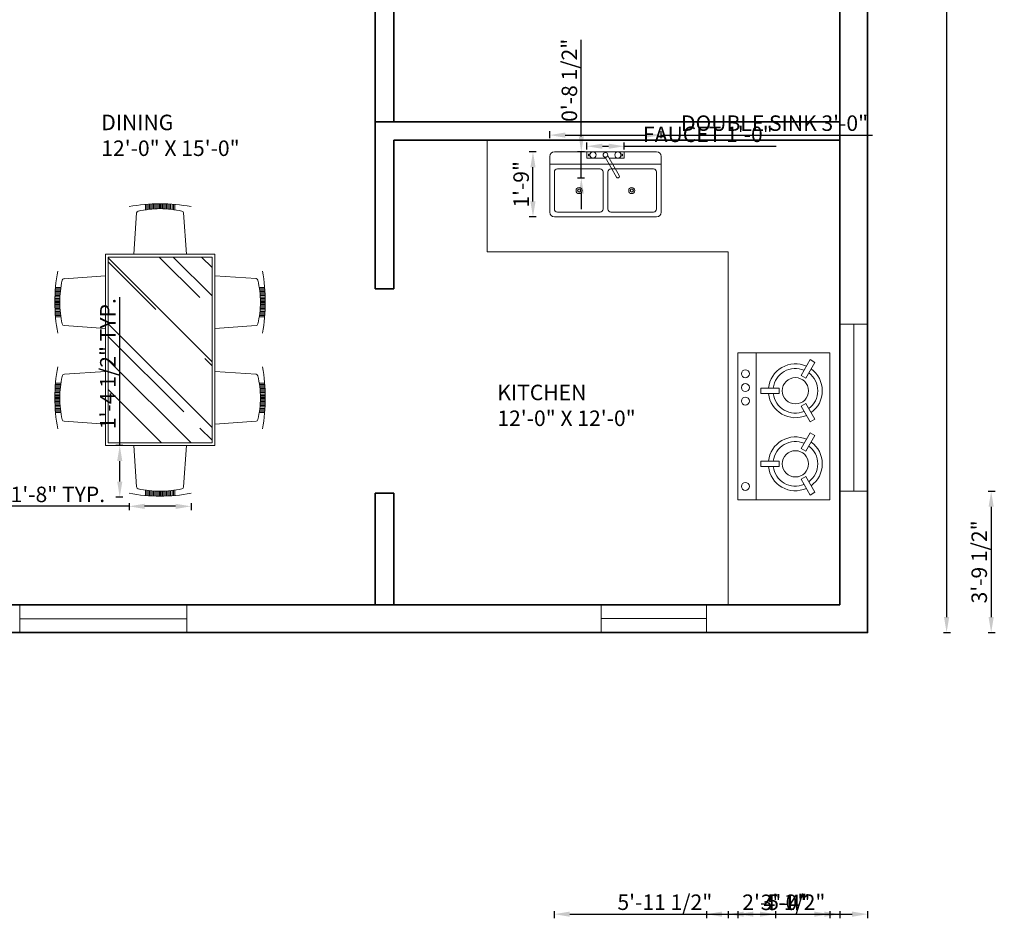
# Model space of a CAD drawing. Units: inches. Extents: x -100 to 766, y -562 to 63.
# Tile 10 of 11: x 448 to 766, y -562 to -269. Entities that reach past the tile are written whole.
import ezdxf

# ---------------------------------------------------------------- set-up
doc = ezdxf.new("R2010")
doc.units = ezdxf.units.IN
for name, color, linetype, lineweight in [('A-ANNO-DIMS', 2, 'Continuous', 18), ('A-AREA-IDEN', 7, 'Continuous', 18), ('A-EQPM', 9, 'Continuous', 18), ('A-FLOR-CASE', 32, 'Continuous', 18), ('A-FLOR-FIXT', 8, 'Continuous', 18), ('A-FURN-PATT', 252, 'Continuous', 13), ('A-GLAZ', 4, 'Continuous', 18), ('A-WALL', 7, 'Continuous', 35), ('furn', 8, 'Continuous', 13)]:
    doc.layers.add(name, color=color, linetype=linetype, lineweight=lineweight)
doc.styles.get("Standard").update_dxf_attribs({"font": 'arial.ttf'})
doc.dimstyles.new('ISO-25', dxfattribs={"dimtxt": 5, "dimasz": 5, "dimexe": 1.25, "dimexo": 0.625, "dimtad": 1, "dimlunit": 3, "dimtxsty": 'Standard', "dimcen": 2.5, "dimadec": 0, "dimazin": 0, "dimtfac": 1, "dimtmove": 0, "dimatfit": 3, "dimfxl": 1, "dimfxlon": 1, "dimarcsym": 0})

# ---------------------------------------------------------------- blocks, each defined once
blk = doc.blocks.new('Sink-double - 36 in top')
for p, q in [((-18, -4), (18, -4)), ((-0.75, -18.5), (-0.75, -6.5)), ((0.75, -6.5), (0.75, -18.5))]:
    blk.add_line(p, q)
for points in [[(-16.5, 0), (16.5, 0)], [(-18, -19.5), (-18, -1.5)], [(18, -1.5), (18, -19.5)], [(-15.5, -5.5), (-1.75, -5.5)], [(1.75, -5.5), (15.5, -5.5)], [(-16.5, -18.5), (-16.5, -6.5)], [(16.5, -6.5), (16.5, -18.5)], [(16.5, -21), (-16.5, -21)], [(-1.75, -19.5), (-15.5, -19.5)], [(15.5, -19.5), (1.75, -19.5)]]:
    blk.add_lwpolyline(points)
for centre, radius in [((-8.5, -12.5), 1), ((-8.5, -12.5), 0.5), ((8.5, -12.5), 1), ((8.5, -12.5), 0.5)]:
    blk.add_circle(centre, radius)
for centre, radius, start, end in [((-16.5, -1.5), 1.5, 90, 180), ((16.5, -1.5), 1.5, 0, 90), ((-15.5, -6.5), 1, 90, 180), ((-1.75, -6.5), 1, 0, 90), ((1.75, -6.5), 1, 90, 180), ((15.5, -6.5), 1, 0, 90), ((-15.5, -18.5), 1, 180, 270), ((-1.75, -18.5), 1, 270, 0), ((1.75, -18.5), 1, 180, 270), ((15.5, -18.5), 1, 270, 0), ((-16.5, -19.5), 1.5, 180, 270), ((16.5, -19.5), 1.5, 270, 0)]:
    blk.add_arc(centre, radius, start, end)
blk = doc.blocks.new('Faucet - kit sink top')
for p, q in [((-5.5, -0.75), (-5.5, -1.25)), ((-4.94278, -0.75), (-5.5, -0.75)), ((-5.5, -1.25), (-4.94278, -1.25)), ((-0.14775, -1.7441), (3.56698, -8.1782)), ((4.43301, -7.6782), (0.71828, -1.2441)), ((4.94278, -0.75), (5.5, -0.75)), ((5.5, -1.25), (4.94278, -1.25)), ((5.5, -0.75), (5.5, -1.25))]:
    blk.add_line(p, q)
blk.add_lwpolyline([(-0.00587, -2), (-6, -2), (-6, 0), (6, 0), (6, -2), (1.15195, -2)])
for centre, radius in [((-4, -1), 1), ((4, -1), 1), ((0, -1), 0.75)]:
    blk.add_circle(centre, radius)
blk.add_arc((4, -7.9282), 0.5, 210, 30)
blk = doc.blocks.new('*D10')
at = {"layer": 'A-ANNO-DIMS', "color": 0, "lineweight": -2, "transparency": 16777216}
for p, q in [((745.89, 12.79), (748.14, 12.79)), ((746.89, 7.79), (746.89, -462.21)), ((745.89, -467.21), (748.14, -467.21))]:
    blk.add_line(p, q, dxfattribs=at)
at = {"layer": 'A-ANNO-DIMS', "color": 0, "transparency": 16777216}
for points in [[(746.06, 7.79), (747.73, 7.79), (746.89, 12.79)], [(746.06, -462.21), (747.73, -462.21), (746.89, -467.21)]]:
    blk.add_solid(points, dxfattribs=at)
at = {"layer": 'Defpoints', "color": 0, "transparency": 16777216}
for p in [(721.39, 12.79), (721.39, -467.21), (746.89, -467.21)]:
    blk.add_point(p, dxfattribs=at)
at = {"layer": 'A-ANNO-DIMS', "color": 0, "transparency": 16777216, "insert": (743.72, -227.21), "char_height": 5, "attachment_point": 5, "rotation": 90}
blk.add_mtext("40'", dxfattribs=at)
blk = doc.blocks.new('WIN-54IN')
blk.add_line((4.5, 54), (4.5, 0))
blk.add_lwpolyline([(0, 54), (9, 54), (9, 0), (0, 0)], close=True)
blk = doc.blocks.new('WIN-34IN')
blk.add_line((4.5, 34), (4.5, 0))
blk.add_lwpolyline([(0, 34), (9, 34), (9, 0), (0, 0)], close=True)
blk = doc.blocks.new('CHAIR-DINING')
for p, q in [((16.31, 18.5), (2.96, 17.59)), ((1.73, 12.99), (0.08, 12.99)), ((1.77, 13.43), (0.11, 13.43)), ((1.83, 13.87), (0.13, 13.87)), ((1.88, 14.32), (0.17, 14.32)), ((1.94, 14.76), (0.2, 14.76)), ((1.56, 10.34), (0, 10.34)), ((1.56, 10.01), (0, 10.01)), ((1.56, 9.68), (0, 9.68)), ((1.6, 11.23), (0.01, 11.23)), ((1.58, 10.79), (0.01, 10.79)), ((1.62, 11.67), (0.02, 11.67)), ((1.65, 12.11), (0.04, 12.11)), ((1.69, 12.55), (0.06, 12.55)), ((1.58, 9.24), (0.01, 9.24)), ((1.6, 8.8), (0.01, 8.8)), ((1.62, 8.36), (0.02, 8.36)), ((1.65, 7.92), (0.04, 7.92)), ((1.69, 7.48), (0.06, 7.48)), ((1.73, 7.04), (0.08, 7.04)), ((1.77, 6.6), (0.11, 6.6)), ((1.83, 6.15), (0.13, 6.15)), ((1.88, 5.71), (0.17, 5.71)), ((1.94, 5.27), (0.2, 5.27)), ((16.31, 1.53), (2.96, 2.43))]:
    blk.add_line(p, q)
blk.add_lwpolyline([(0.91, 20.03, 0.091245), (0.91, 0, 0.091245)], format="xyb")
for centre, radius, start, end in [((38.68, 9.38), 37.13, 168.0355, 179.0138), ((3.01, 16.93), 0.662, 93.8745, 168.0355), ((38.68, 10.65), 37.13, 180.9862, 191.9645), ((3.01, 3.09), 0.662, 191.9645, 266.1255)]:
    blk.add_arc(centre, radius, start, end)
blk = doc.blocks.new('*D24')
at = {"layer": 'A-ANNO-DIMS', "color": 0, "lineweight": -2, "transparency": 16777216}
for p, q in [((482.94, -425.44), (482.94, -427.69)), ((502.97, -425.44), (502.97, -427.69)), ((482.94, -426.44), (404.32, -426.44)), ((497.97, -426.44), (487.94, -426.44))]:
    blk.add_line(p, q, dxfattribs=at)
at = {"layer": 'A-ANNO-DIMS', "color": 0, "transparency": 16777216}
for points in [[(487.94, -425.61), (487.94, -427.28), (482.94, -426.44)], [(497.97, -425.61), (497.97, -427.28), (502.97, -426.44)]]:
    blk.add_solid(points, dxfattribs=at)
at = {"layer": 'Defpoints', "color": 0, "transparency": 16777216}
for p in [(482.94, -423.44), (502.97, -423.44), (482.94, -426.44)]:
    blk.add_point(p, dxfattribs=at)
at = {"layer": 'A-ANNO-DIMS', "color": 0, "transparency": 16777216, "insert": (441.13, -423.23), "char_height": 5, "attachment_point": 5, "rotation": 0}
blk.add_mtext('SIDE CHAIR 1\'-8" TYP.', dxfattribs=at)
blk = doc.blocks.new('*D25')
at = {"layer": 'A-ANNO-DIMS', "color": 0, "lineweight": -2, "transparency": 16777216}
for p, q in [((479.93, -406.82), (479.93, -358.91)), ((480.93, -406.82), (478.68, -406.82)), ((479.93, -418.44), (479.93, -411.82)), ((480.93, -423.44), (478.68, -423.44))]:
    blk.add_line(p, q, dxfattribs=at)
at = {"layer": 'A-ANNO-DIMS', "color": 0, "transparency": 16777216}
for points in [[(479.1, -411.82), (480.77, -411.82), (479.93, -406.82)], [(479.1, -418.44), (480.77, -418.44), (479.93, -423.44)]]:
    blk.add_solid(points, dxfattribs=at)
at = {"layer": 'Defpoints', "color": 0, "transparency": 16777216}
for p in [(479.93, -406.82), (482.94, -406.82), (482.94, -423.44)]:
    blk.add_point(p, dxfattribs=at)
at = {"layer": 'A-ANNO-DIMS', "color": 0, "transparency": 16777216, "insert": (476.72, -380.37), "char_height": 5, "attachment_point": 5, "rotation": 90}
blk.add_mtext('1\'-4 1/2" TYP.', dxfattribs=at)
blk = doc.blocks.new('*D36')
at = {"layer": 'A-ANNO-DIMS', "color": 0, "lineweight": -2, "transparency": 16777216}
for p, q in [((630.75, -311.15), (630.75, -308.9)), ((635.75, -310.15), (637.75, -310.15)), ((642.75, -311.15), (642.75, -308.9)), ((642.75, -310.15), (691.89, -310.15))]:
    blk.add_line(p, q, dxfattribs=at)
at = {"layer": 'A-ANNO-DIMS', "color": 0, "transparency": 16777216}
for points in [[(635.75, -309.31), (635.75, -310.98), (630.75, -310.15)], [(637.75, -309.31), (637.75, -310.98), (642.75, -310.15)]]:
    blk.add_solid(points, dxfattribs=at)
at = {"layer": 'Defpoints', "color": 0, "transparency": 16777216}
for p in [(642.75, -310.15), (630.75, -311.95), (642.75, -311.95)]:
    blk.add_point(p, dxfattribs=at)
at = {"layer": 'A-ANNO-DIMS', "color": 0, "transparency": 16777216, "insert": (669.82, -306.94), "char_height": 5, "attachment_point": 5}
blk.add_mtext('FAUCET 1\'-0"', dxfattribs=at)
blk = doc.blocks.new('*D37')
at = {"layer": 'A-ANNO-DIMS', "color": 0, "lineweight": -2, "transparency": 16777216}
for p, q in [((628.95, -306.95), (628.95, -275.75)), ((629.95, -311.95), (627.7, -311.95)), ((628.95, -320.45), (628.95, -311.95)), ((629.95, -320.45), (627.7, -320.45)), ((628.95, -325.45), (628.95, -330.45))]:
    blk.add_line(p, q, dxfattribs=at)
at = {"layer": 'A-ANNO-DIMS', "color": 0, "transparency": 16777216}
for points in [[(628.12, -306.95), (629.78, -306.95), (628.95, -311.95)], [(628.12, -325.45), (629.78, -325.45), (628.95, -320.45)]]:
    blk.add_solid(points, dxfattribs=at)
at = {"layer": 'Defpoints', "color": 0, "transparency": 16777216}
for p in [(628.95, -311.95), (630.75, -311.95), (630.75, -320.45)]:
    blk.add_point(p, dxfattribs=at)
at = {"layer": 'A-ANNO-DIMS', "color": 0, "transparency": 16777216, "insert": (625.74, -288.85), "char_height": 5, "attachment_point": 5, "rotation": 90}
blk.add_mtext('0\'-8 1/2"', dxfattribs=at)
blk = doc.blocks.new('*D38')
at = {"layer": 'A-ANNO-DIMS', "color": 0, "lineweight": -2, "transparency": 16777216}
for p, q in [((618.75, -307.55), (618.75, -305.3)), ((623.75, -306.55), (649.75, -306.55)), ((654.75, -307.55), (654.75, -305.3)), ((654.75, -306.55), (722.95, -306.55))]:
    blk.add_line(p, q, dxfattribs=at)
at = {"layer": 'A-ANNO-DIMS', "color": 0, "transparency": 16777216}
for points in [[(623.75, -305.71), (623.75, -307.38), (618.75, -306.55)], [(649.75, -305.71), (649.75, -307.38), (654.75, -306.55)]]:
    blk.add_solid(points, dxfattribs=at)
at = {"layer": 'Defpoints', "color": 0, "transparency": 16777216}
for p in [(654.75, -306.55), (618.75, -311.95), (654.75, -311.95)]:
    blk.add_point(p, dxfattribs=at)
at = {"layer": 'A-ANNO-DIMS', "color": 0, "transparency": 16777216, "insert": (691.35, -303.33), "char_height": 5, "attachment_point": 5}
blk.add_mtext('DOUBLE SINK 3\'-0"', dxfattribs=at)
blk = doc.blocks.new('*D39')
at = {"layer": 'A-ANNO-DIMS', "color": 0, "lineweight": -2, "transparency": 16777216}
for p, q in [((614.35, -311.95), (612.1, -311.95)), ((613.35, -327.95), (613.35, -316.95)), ((614.35, -332.95), (612.1, -332.95))]:
    blk.add_line(p, q, dxfattribs=at)
at = {"layer": 'A-ANNO-DIMS', "color": 0, "transparency": 16777216}
for points in [[(612.52, -316.95), (614.18, -316.95), (613.35, -311.95)], [(612.52, -327.95), (614.18, -327.95), (613.35, -332.95)]]:
    blk.add_solid(points, dxfattribs=at)
at = {"layer": 'Defpoints', "color": 0, "transparency": 16777216}
for p in [(613.35, -311.95), (618.75, -311.95), (618.75, -332.95)]:
    blk.add_point(p, dxfattribs=at)
at = {"layer": 'A-ANNO-DIMS', "color": 0, "transparency": 16777216, "insert": (610.17, -322.45), "char_height": 5, "attachment_point": 5, "rotation": 90}
blk.add_mtext('1\'-9"', dxfattribs=at)
blk = doc.blocks.new('*D49')
at = {"layer": 'A-ANNO-DIMS', "color": 0, "lineweight": -2, "transparency": 16777216}
for p, q in [((-88.51, -356.21), (-90.76, -356.21)), ((-89.51, -361.21), (-89.51, -417.21)), ((-88.51, -422.21), (-90.76, -422.21))]:
    blk.add_line(p, q, dxfattribs=at)
at = {"layer": 'A-ANNO-DIMS', "color": 0, "transparency": 16777216}
for points in [[(-90.35, -361.21), (-88.68, -361.21), (-89.51, -356.21)], [(-90.35, -417.21), (-88.68, -417.21), (-89.51, -422.21)]]:
    blk.add_solid(points, dxfattribs=at)
at = {"layer": 'Defpoints', "color": 0, "transparency": 16777216}
for p in [(562.39, -356.21), (-89.51, -422.21), (562.39, -422.21)]:
    blk.add_point(p, dxfattribs=at)
at = {"layer": 'A-ANNO-DIMS', "color": 0, "transparency": 16777216, "insert": (-92.69, -389.21), "char_height": 5, "attachment_point": 5, "rotation": 90}
blk.add_mtext('5\'-6"', dxfattribs=at)
blk = doc.blocks.new('*D50')
at = {"layer": 'A-ANNO-DIMS', "color": 0, "lineweight": -2, "transparency": 16777216}
for p, q in [((676.39, -557.16), (676.39, -559.41)), ((681.39, -558.16), (707.39, -558.16)), ((712.39, -557.16), (712.39, -559.41))]:
    blk.add_line(p, q, dxfattribs=at)
at = {"layer": 'A-ANNO-DIMS', "color": 0, "transparency": 16777216}
for points in [[(681.39, -557.32), (681.39, -558.99), (676.39, -558.16)], [(707.39, -557.32), (707.39, -558.99), (712.39, -558.16)]]:
    blk.add_solid(points, dxfattribs=at)
at = {"layer": 'Defpoints', "color": 0, "transparency": 16777216}
for p in [(676.39, -458.21), (712.39, -458.21), (712.39, -558.16)]:
    blk.add_point(p, dxfattribs=at)
at = {"layer": 'A-ANNO-DIMS', "color": 0, "transparency": 16777216, "insert": (694.39, -554.98), "char_height": 5, "attachment_point": 5}
blk.add_mtext('3\'-0"', dxfattribs=at)
blk = doc.blocks.new('*D51')
at = {"layer": 'A-ANNO-DIMS', "color": 0, "lineweight": -2, "transparency": 16777216}
for p, q in [((-88.51, -308.21), (-90.76, -308.21)), ((-89.51, -313.21), (-89.51, -339.21)), ((-88.51, -344.21), (-90.76, -344.21))]:
    blk.add_line(p, q, dxfattribs=at)
at = {"layer": 'A-ANNO-DIMS', "color": 0, "transparency": 16777216}
for points in [[(-90.35, -313.21), (-88.68, -313.21), (-89.51, -308.21)], [(-90.35, -339.21), (-88.68, -339.21), (-89.51, -344.21)]]:
    blk.add_solid(points, dxfattribs=at)
at = {"layer": 'Defpoints', "color": 0, "transparency": 16777216}
for p in [(598.6, -308.21), (-89.51, -344.21), (598.6, -344.21)]:
    blk.add_point(p, dxfattribs=at)
at = {"layer": 'A-ANNO-DIMS', "color": 0, "transparency": 16777216, "insert": (-92.69, -326.21), "char_height": 5, "attachment_point": 5, "rotation": 90}
blk.add_mtext('3\'-0"', dxfattribs=at)
blk = doc.blocks.new('*D52')
at = {"layer": 'A-ANNO-DIMS', "color": 0, "lineweight": -2, "transparency": 16777216}
for p, q in [((568.39, 51.68), (568.39, 53.93)), ((573.39, 52.68), (593.6, 52.68)), ((598.6, 51.68), (598.6, 53.93))]:
    blk.add_line(p, q, dxfattribs=at)
at = {"layer": 'A-ANNO-DIMS', "color": 0, "transparency": 16777216}
for points in [[(573.39, 53.51), (573.39, 51.84), (568.39, 52.68)], [(593.6, 53.51), (593.6, 51.84), (598.6, 52.68)]]:
    blk.add_solid(points, dxfattribs=at)
at = {"layer": 'Defpoints', "color": 0, "transparency": 16777216}
for p in [(598.6, 52.68), (568.39, -308.21), (598.6, -308.21)]:
    blk.add_point(p, dxfattribs=at)
at = {"layer": 'A-ANNO-DIMS', "color": 0, "transparency": 16777216, "insert": (583.5, 55.86), "char_height": 5, "attachment_point": 5}
blk.add_mtext('2\'-6"', dxfattribs=at)
blk = doc.blocks.new('*D64')
at = {"layer": 'A-ANNO-DIMS', "color": 0, "lineweight": -2, "transparency": 16777216}
for p, q in [((760.28, -421.57), (762.53, -421.57)), ((761.28, -426.57), (761.28, -462.21)), ((760.28, -467.21), (762.53, -467.21))]:
    blk.add_line(p, q, dxfattribs=at)
at = {"layer": 'A-ANNO-DIMS', "color": 0, "transparency": 16777216}
for points in [[(760.45, -426.57), (762.11, -426.57), (761.28, -421.57)], [(760.45, -462.21), (762.11, -462.21), (761.28, -467.21)]]:
    blk.add_solid(points, dxfattribs=at)
at = {"layer": 'Defpoints', "color": 0, "transparency": 16777216}
for p in [(721.39, -421.57), (721.39, -467.21), (761.28, -467.21)]:
    blk.add_point(p, dxfattribs=at)
at = {"layer": 'A-ANNO-DIMS', "color": 0, "transparency": 16777216, "insert": (758.07, -444.39), "char_height": 5, "attachment_point": 5, "rotation": 90}
blk.add_mtext('3\'-9 1/2"', dxfattribs=at)
blk = doc.blocks.new('*D69')
at = {"layer": 'A-ANNO-DIMS', "color": 0, "lineweight": -2, "transparency": 16777216}
for p, q in [((669.37, -557.16), (669.37, -559.41)), ((674.37, -558.16), (716.39, -558.16)), ((721.39, -557.16), (721.39, -559.41))]:
    blk.add_line(p, q, dxfattribs=at)
at = {"layer": 'A-ANNO-DIMS', "color": 0, "transparency": 16777216}
for points in [[(674.37, -557.32), (674.37, -558.99), (669.37, -558.16)], [(716.39, -557.32), (716.39, -558.99), (721.39, -558.16)]]:
    blk.add_solid(points, dxfattribs=at)
at = {"layer": 'Defpoints', "color": 0, "transparency": 16777216}
for p in [(669.37, -467.21), (721.39, -467.21), (721.39, -558.16)]:
    blk.add_point(p, dxfattribs=at)
at = {"layer": 'A-ANNO-DIMS', "color": 0, "transparency": 16777216, "insert": (695.38, -555.03), "char_height": 5, "attachment_point": 5}
blk.add_mtext('4\'-4"', dxfattribs=at)
blk = doc.blocks.new('*D70')
at = {"layer": 'A-ANNO-DIMS', "color": 0, "lineweight": -2, "transparency": 16777216}
for p, q in [((-88.51, -376.85), (-90.76, -376.85)), ((-89.51, -381.85), (-89.51, -419.34)), ((-88.51, -424.34), (-90.76, -424.34))]:
    blk.add_line(p, q, dxfattribs=at)
at = {"layer": 'A-ANNO-DIMS', "color": 0, "transparency": 16777216}
for points in [[(-90.35, -381.85), (-88.68, -381.85), (-89.51, -376.85)], [(-90.35, -419.34), (-88.68, -419.34), (-89.51, -424.34)]]:
    blk.add_solid(points, dxfattribs=at)
at = {"layer": 'Defpoints', "color": 0, "transparency": 16777216}
for p in [(679.5, -376.85), (-89.51, -424.34), (679.5, -424.34)]:
    blk.add_point(p, dxfattribs=at)
at = {"layer": 'A-ANNO-DIMS', "color": 0, "transparency": 16777216, "insert": (-92.73, -400.59), "char_height": 5, "attachment_point": 5, "rotation": 90}
blk.add_mtext('3\'-11 1/2"', dxfattribs=at)
blk = doc.blocks.new('*D71')
at = {"layer": 'A-ANNO-DIMS', "color": 0, "lineweight": -2, "transparency": 16777216}
for p, q in [((679.5, -557.16), (679.5, -559.41)), ((684.5, -558.16), (704.17, -558.16)), ((709.17, -557.16), (709.17, -559.41))]:
    blk.add_line(p, q, dxfattribs=at)
at = {"layer": 'A-ANNO-DIMS', "color": 0, "transparency": 16777216}
for points in [[(684.5, -557.32), (684.5, -558.99), (679.5, -558.16)], [(704.17, -557.32), (704.17, -558.99), (709.17, -558.16)]]:
    blk.add_solid(points, dxfattribs=at)
at = {"layer": 'Defpoints', "color": 0, "transparency": 16777216}
for p in [(679.5, -424.34), (709.17, -424.34), (709.17, -558.16)]:
    blk.add_point(p, dxfattribs=at)
at = {"layer": 'A-ANNO-DIMS', "color": 0, "transparency": 16777216, "insert": (694.34, -554.95), "char_height": 5, "attachment_point": 5}
blk.add_mtext('2\'-5 1/2"', dxfattribs=at)
blk = doc.blocks.new('*D72')
at = {"layer": 'A-ANNO-DIMS', "color": 0, "lineweight": -2, "transparency": 16777216}
for p, q in [((475.3, 51.68), (475.3, 53.93)), ((480.3, 52.68), (505.6, 52.68)), ((510.6, 51.68), (510.6, 53.93))]:
    blk.add_line(p, q, dxfattribs=at)
at = {"layer": 'A-ANNO-DIMS', "color": 0, "transparency": 16777216}
for points in [[(480.3, 53.51), (480.3, 51.84), (475.3, 52.68)], [(505.6, 53.51), (505.6, 51.84), (510.6, 52.68)]]:
    blk.add_solid(points, dxfattribs=at)
at = {"layer": 'Defpoints', "color": 0, "transparency": 16777216}
for p in [(510.6, 52.68), (475.3, -345.04), (510.6, -345.04)]:
    blk.add_point(p, dxfattribs=at)
at = {"layer": 'A-ANNO-DIMS', "color": 0, "transparency": 16777216, "insert": (492.95, 55.89), "char_height": 5, "attachment_point": 5}
blk.add_mtext('2\'-11 1/2"', dxfattribs=at)
blk = doc.blocks.new('*D73')
at = {"layer": 'A-ANNO-DIMS', "color": 0, "lineweight": -2, "transparency": 16777216}
for p, q in [((-88.51, -345.04), (-90.76, -345.04)), ((-89.51, -350.04), (-89.51, -401.82)), ((-88.51, -406.82), (-90.76, -406.82))]:
    blk.add_line(p, q, dxfattribs=at)
at = {"layer": 'A-ANNO-DIMS', "color": 0, "transparency": 16777216}
for points in [[(-90.35, -350.04), (-88.68, -350.04), (-89.51, -345.04)], [(-90.35, -401.82), (-88.68, -401.82), (-89.51, -406.82)]]:
    blk.add_solid(points, dxfattribs=at)
at = {"layer": 'Defpoints', "color": 0, "transparency": 16777216}
for p in [(475.3, -345.04), (-89.51, -406.82), (475.3, -406.82)]:
    blk.add_point(p, dxfattribs=at)
at = {"layer": 'A-ANNO-DIMS', "color": 0, "transparency": 16777216, "insert": (-92.69, -375.93), "char_height": 5, "attachment_point": 5, "rotation": 90}
blk.add_mtext('5\'-2"', dxfattribs=at)
blk = doc.blocks.new('*D74')
at = {"layer": 'A-ANNO-DIMS', "color": 0, "lineweight": -2, "transparency": 16777216}
for p, q in [((620.21, -557.16), (620.21, -559.41)), ((625.21, -558.16), (686.63, -558.16)), ((691.63, -557.16), (691.63, -559.41))]:
    blk.add_line(p, q, dxfattribs=at)
at = {"layer": 'A-ANNO-DIMS', "color": 0, "transparency": 16777216}
for points in [[(625.21, -557.32), (625.21, -558.99), (620.21, -558.16)], [(686.63, -557.32), (686.63, -558.99), (691.63, -558.16)]]:
    blk.add_solid(points, dxfattribs=at)
at = {"layer": 'Defpoints', "color": 0, "transparency": 16777216}
for p in [(620.21, -98.08), (691.63, -98.08), (691.63, -558.16)]:
    blk.add_point(p, dxfattribs=at)
at = {"layer": 'A-ANNO-DIMS', "color": 0, "transparency": 16777216, "insert": (655.92, -554.95), "char_height": 5, "attachment_point": 5}
blk.add_mtext('5\'-11 1/2"', dxfattribs=at)
blk = doc.blocks.new('*D83')
at = {"layer": 'A-ANNO-DIMS', "color": 0, "lineweight": -2, "transparency": 16777216}
for p, q in [((-88.51, -422.21), (-90.76, -422.21)), ((-89.51, -427.21), (-89.51, -453.21)), ((-88.51, -458.21), (-90.76, -458.21))]:
    blk.add_line(p, q, dxfattribs=at)
at = {"layer": 'A-ANNO-DIMS', "color": 0, "transparency": 16777216}
for points in [[(-90.35, -427.21), (-88.68, -427.21), (-89.51, -422.21)], [(-90.35, -453.21), (-88.68, -453.21), (-89.51, -458.21)]]:
    blk.add_solid(points, dxfattribs=at)
at = {"layer": 'Defpoints', "color": 0, "transparency": 16777216}
for p in [(562.39, -422.21), (-89.51, -458.21), (562.39, -458.21)]:
    blk.add_point(p, dxfattribs=at)
at = {"layer": 'A-ANNO-DIMS', "color": 0, "transparency": 16777216, "insert": (-92.69, -440.21), "char_height": 5, "attachment_point": 5, "rotation": 90}
blk.add_mtext('3\'-0"', dxfattribs=at)

msp = doc.modelspace()

# ---------------------------------------------------------------- hatches: boundary and pattern name
at = {"layer": 'A-FURN-PATT'}
h = msp.add_hatch(dxfattribs=at)
h.set_pattern_fill('AR-RROOF', color=256, scale=0.882529, angle=-45, style=0)
h.set_pattern_definition([(315, (-259.83, 1276.079), (50.72213, -19.0208), [336.2434, -44.8325, 112.0811, -22.4162]), (315, (-230.824, 1262.923), (5.2307, 36.93205), [67.2487, -7.3974, 134.4974, -16.8122]), (315, (-238.432, 1281.626), (93.04341, -71.80352), [179.3298, -31.3827, 89.6649, -22.4162])])
h.paths.add_polyline_path([(509.719, -345.927), (476.183, -345.927), (476.183, -405.939), (509.719, -405.939)])

# ---------------------------------------------------------------- linework, layer by layer
at = {"layer": 'A-EQPM'}
for p, q in [((679.495, -424.336), (679.495, -376.848)), ((679.495, -376.848), (709.175, -376.848)), ((685.431, -424.336), (685.431, -376.848)), ((709.175, -424.336), (709.175, -376.848)), ((699.899, -384.177), (702.859, -379.055)), ((701.441, -385.068), (704.401, -379.946)), ((702.859, -379.055), (704.401, -379.946)), ((699.899, -384.177), (701.441, -385.068)), ((686.958, -390.008), (686.959, -388.227)), ((692.873, -390.01), (686.958, -390.008)), ((692.874, -388.229), (686.959, -388.227)), ((692.873, -390.01), (692.874, -388.229)), ((701.438, -393.178), (699.896, -394.068)), ((699.896, -394.068), (702.852, -399.192)), ((701.438, -393.178), (704.394, -398.302)), ((704.394, -398.302), (702.852, -399.192)), ((699.899, -407.776), (702.859, -402.654)), ((701.441, -408.667), (704.401, -403.545)), ((702.859, -402.654), (704.401, -403.545)), ((699.899, -407.776), (701.441, -408.667)), ((686.958, -413.607), (686.959, -411.826)), ((692.874, -411.828), (686.959, -411.826)), ((692.873, -413.609), (692.874, -411.828)), ((692.873, -413.609), (686.958, -413.607)), ((701.438, -416.777), (699.896, -417.667)), ((699.896, -417.667), (702.852, -422.791)), ((701.438, -416.777), (704.394, -421.901)), ((704.394, -421.901), (702.852, -422.791)), ((679.495, -424.336), (709.175, -424.336))]:
    msp.add_line(p, q, dxfattribs=at)
at = {"layer": 'A-EQPM', "extrusion": (0, 0, -1)}
for centre, major_axis, start_param, end_param in [((698.07, -389.121), (8.697, 0.005), 3.2450997, 5.1343764), ((681.926, -383.607), (0.911, 0.911), 2.3561945, 8.6393798), ((698.07, -389.121), (5.1, 5.1), 4.0511235, 5.8980015), ((698.07, -389.121), (3.002, 3.002), 2.3561945, 8.6393798), ((698.07, -389.121), (5.1, 5.1), 6.1455186, 7.9923966), ((698.07, -389.121), (8.697, 0.015), -0.9425843, 0.9466925), ((681.926, -388.069), (0.911, 0.911), 2.3561945, 8.6393798), ((698.07, -389.121), (8.697, -0.012), 1.148752, 3.0380287), ((698.07, -389.121), (5.1, -5.1), 0.385932, 2.2328101), ((681.926, -392.432), (0.911, 0.911), 2.3561945, 8.6393798), ((698.07, -412.721), (8.697, -0.003), 3.2441732, 5.1334499), ((698.07, -412.721), (5.1, -5.1), 2.4803271, 4.3272052), ((698.07, -412.721), (8.697, 0.002), -0.9440105, 0.9452662), ((698.07, -412.721), (3.002, 3.002), 2.3561945, 8.6393798), ((698.07, -412.721), (5.1, 5.1), 6.1455186, 7.9923966), ((698.07, -412.721), (8.697, -0.012), 1.1487904, 3.0380671), ((698.07, -412.721), (5.1, -5.1), 0.385932, 2.2328101), ((681.926, -419.997), (0.911, 0.911), 2.3561945, 8.6393798)]:
    msp.add_ellipse(centre, major_axis=major_axis, ratio=1, start_param=start_param, end_param=end_param, dxfattribs=at)
at = {"layer": 'A-FLOR-CASE'}
for p, q in [((598.603, -344.214), (598.603, -308.214)), ((598.603, -344.214), (676.388, -344.214)), ((676.388, -458.214), (676.388, -344.214))]:
    msp.add_line(p, q, dxfattribs=at)
at = {"layer": 'A-WALL'}
for p, q in [((712.388, 3.786), (712.388, -458.214)), ((562.394, -302.214), (562.394, -257.081)), ((568.394, -302.214), (568.394, -257.214)), ((562.394, -306.262), (562.394, -302.214)), ((568.394, -302.214), (562.394, -302.214)), ((712.388, -302.214), (568.394, -302.214)), ((562.394, -312.262), (562.394, -306.262)), ((712.388, -308.214), (568.394, -308.214)), ((568.394, -356.214), (568.394, -308.214)), ((562.394, -356.214), (562.394, -312.262)), ((568.394, -356.214), (562.394, -356.214)), ((562.394, -458.214), (562.394, -422.214)), ((568.394, -422.214), (562.394, -422.214)), ((568.394, -458.214), (568.394, -422.214)), ((532.388, -458.214), (250.388, -458.214)), ((568.394, -458.214), (532.388, -458.214)), ((712.388, -458.214), (568.394, -458.214))]:
    msp.add_line(p, q, dxfattribs=at)
msp.add_lwpolyline([(1.388, 12.786), (721.388, 12.786), (721.388, -467.214), (1.388, -467.214)], close=True, dxfattribs=at)
at = {"layer": 'furn'}
for p, q in [((475.3, -382.892), (462.115, -383.785)), ((460.813, -387.517), (459.122, -387.517)), ((460.869, -387.076), (459.154, -387.076)), ((460.931, -386.635), (459.191, -386.635)), ((460.566, -390.606), (458.992, -390.606)), ((460.585, -390.165), (459, -390.165)), ((460.61, -389.724), (459.012, -389.724)), ((460.64, -389.283), (459.027, -389.283)), ((460.675, -388.841), (459.045, -388.841)), ((460.716, -388.4), (459.067, -388.4)), ((460.762, -387.959), (459.093, -387.959)), ((460.545, -391.377), (458.987, -391.377)), ((460.552, -391.048), (458.988, -391.048)), ((460.552, -391.707), (458.988, -391.707)), ((460.566, -392.149), (458.992, -392.149)), ((460.585, -392.59), (459, -392.59)), ((460.61, -393.031), (459.012, -393.031)), ((460.64, -393.472), (459.027, -393.472)), ((460.675, -393.914), (459.045, -393.914)), ((460.716, -394.355), (459.067, -394.355)), ((460.762, -394.796), (459.093, -394.796)), ((460.813, -395.237), (459.122, -395.237)), ((460.869, -395.679), (459.154, -395.679)), ((460.931, -396.12), (459.191, -396.12)), ((475.3, -399.863), (461.949, -398.958))]:
    msp.add_line(p, q, dxfattribs=at)
for points in [[(475.3, -345.045), (475.3, -406.822), (510.601, -406.822), (510.601, -345.045)], [(476.183, -345.927), (476.183, -405.939), (509.719, -405.939), (509.719, -345.927)]]:
    msp.add_lwpolyline(points, close=True, dxfattribs=at)
msp.add_lwpolyline([(459.901, -401.392, -0.0912453), (459.901, -381.363, -0.0912453)], format="xyb", dxfattribs=at)
for centre, radius, start, end in [((497.666, -392.016), 37.127, 168.29889, 179.01382), ((462.175, -384.666), 0.883, 93.87448, 168.29889), ((497.666, -390.738), 37.127, 180.98618, 191.96453), ((461.993, -398.298), 0.662, 191.96453, 266.12552)]:
    msp.add_arc(centre, radius, start, end, dxfattribs=at)

# ---------------------------------------------------------------- block references
at = {"layer": 'A-FLOR-FIXT'}
for name in ['Sink-double - 36 in top', 'Faucet - kit sink top']:
    msp.add_blockref(name, (636.751, -311.946), dxfattribs=at)
at = {"layer": 'A-GLAZ'}
msp.add_blockref('WIN-54IN', (712.388, -421.575), dxfattribs=at)
at = {"layer": 'A-GLAZ', "rotation": 270}
for name, p in [('WIN-54IN', (447.624, -458.288)), ('WIN-34IN', (635.368, -458.215))]:
    msp.add_blockref(name, p, dxfattribs=at)
at = {"layer": 'furn'}
for p, rotation in [((482.937, -328.731), 270.000000003954), ((526.915, -350.475), 180), ((526.915, -381.363), 180), ((502.965, -423.135), 90.0000000036786)]:
    msp.add_blockref('CHAIR-DINING', p, dxfattribs=dict(at, rotation=rotation))
msp.add_blockref('CHAIR-DINING', (458.987, -370.503), dxfattribs=at)

# ---------------------------------------------------------------- texts
at = {"layer": 'A-AREA-IDEN', "char_height": 5, "attachment_point": 1}
for s, width, insert in [('DINING\\P12\'-0" X 15\'-0"', 59.99417, (473.963, -299.954)), ('KITCHEN\\P12\'-0" X 12\'-0"', 54.88458, (601.839, -387.165))]:
    msp.add_mtext_dynamic_manual_height_columns(s, width=width, gutter_width=12.5, heights=[0], dxfattribs=dict(at, insert=insert))

# ---------------------------------------------------------------- dimensions: what is measured, and where the dimension line sits
at = {"layer": 'A-ANNO-DIMS'}
for base, p1, p2, picture, middle in [((510.601, 52.678), (475.3, -345.045), (510.601, -345.045), '*D72', (492.951, 55.888)), ((598.603, 52.678), (568.394, -308.214), (598.603, -308.214), '*D52', (583.499, 55.855)), ((691.632, -558.156), (620.215, -98.077), (691.632, -98.077), '*D74', (655.923, -554.946)), ((709.175, -558.156), (679.495, -424.336), (709.175, -424.336), '*D71', (694.335, -554.946)), ((712.388, -558.156), (676.388, -458.214), (712.388, -458.214), '*D50', (694.388, -554.977)), ((721.388, -558.156), (669.368, -467.214), (721.388, -467.214), '*D69', (695.378, -555.031))]:
    dim = msp.add_linear_dim(base=base, p1=p1, p2=p2, dimstyle='ISO-25', override={"dimdec": 1, "dimlfac": 1, "dimrnd": 0, "dimzin": 1, "dimdsep": 46, "dimlunit": 4, "dimfrac": 2}, dxfattribs=at)
    dim.commit()
    dim.dimension.update_dxf_attribs({"geometry": picture, "text_midpoint": middle})
for base, p1, p2, override, picture, middle in [((746.895, -467.214), (721.388, 12.786), (721.388, -467.214), {"dimclrd": 0, "dimclre": 0, "dimclrt": 0}, '*D10', (743.717, -227.214)), ((628.951, -311.946), (630.751, -320.445), (630.751, -311.946), {"dimdec": 1, "dimlfac": 1, "dimrnd": 0, "dimzin": 1, "dimdsep": 46, "dimlunit": 4, "dimfrac": 2}, '*D37', (625.741, -288.85)), ((-89.513, -344.214), (598.603, -308.214), (598.603, -344.214), {"dimdec": 1, "dimlfac": 1, "dimrnd": 0, "dimzin": 1, "dimdsep": 46, "dimlunit": 4, "dimfrac": 2}, '*D51', (-92.693, -326.214)), ((613.351, -311.946), (618.751, -332.946), (618.751, -311.946), {"dimdec": 1, "dimlfac": 1, "dimrnd": 0, "dimzin": 1, "dimdsep": 46, "dimlunit": 4, "dimfrac": 2}, '*D39', (610.173, -322.446)), ((-89.513, -406.822), (475.3, -345.045), (475.3, -406.822), {"dimdec": 1, "dimlfac": 1, "dimrnd": 0, "dimzin": 1, "dimdsep": 46, "dimlunit": 4, "dimfrac": 2}, '*D73', (-92.691, -375.933)), ((-89.513, -422.214), (562.394, -356.214), (562.394, -422.214), {"dimdec": 1, "dimlfac": 1, "dimrnd": 0, "dimzin": 1, "dimdsep": 46, "dimlunit": 4, "dimfrac": 2}, '*D49', (-92.691, -389.214)), ((-89.513, -424.336), (679.495, -376.848), (679.495, -424.336), {"dimdec": 1, "dimlfac": 1, "dimrnd": 0, "dimzin": 1, "dimdsep": 46, "dimlunit": 4, "dimfrac": 2}, '*D70', (-92.725, -400.592)), ((-89.513, -458.214), (562.394, -422.214), (562.394, -458.214), {"dimdec": 1, "dimlfac": 1, "dimrnd": 0, "dimzin": 1, "dimdsep": 46, "dimlunit": 4, "dimfrac": 2}, '*D83', (-92.693, -440.214)), ((761.28, -467.214), (721.388, -421.575), (721.388, -467.214), {"dimdec": 1, "dimlfac": 1, "dimrnd": 0, "dimzin": 1, "dimdsep": 46, "dimlunit": 4, "dimfrac": 2}, '*D64', (758.068, -444.395))]:
    dim = msp.add_linear_dim(base=base, p1=p1, p2=p2, angle=90, dimstyle='ISO-25', override=override, dxfattribs=at)
    dim.commit()
    dim.dimension.update_dxf_attribs({"geometry": picture, "text_midpoint": middle})
for base, p1, p2, text, picture, middle in [((654.751, -306.546), (618.751, -311.946), (654.751, -311.946), 'DOUBLE SINK <>', '*D38', (691.352, -303.332)), ((642.751, -310.146), (630.751, -311.946), (642.751, -311.946), 'FAUCET <>', '*D36', (669.821, -306.936))]:
    dim = msp.add_linear_dim(base=base, p1=p1, p2=p2, text=text, dimstyle='ISO-25', override={"dimdec": 1, "dimlfac": 1, "dimrnd": 0, "dimzin": 1, "dimdsep": 46, "dimlunit": 4, "dimfrac": 2}, dxfattribs=at)
    dim.commit()
    dim.dimension.update_dxf_attribs({"geometry": picture, "text_midpoint": middle})
for base, p1, p2, angle, text, picture, middle in [((479.932, -406.822), (482.936, -423.44), (482.936, -406.822), 90, '<> TYP.', '*D25', (476.722, -380.368)), ((482.936, -426.444), (502.965, -423.44), (482.936, -423.44), 180, 'SIDE CHAIR <> TYP.', '*D24', (441.126, -423.234))]:
    dim = msp.add_linear_dim(base=base, p1=p1, p2=p2, angle=angle, text=text, dimstyle='ISO-25', override={"dimdec": 1, "dimlfac": 1, "dimrnd": 0, "dimzin": 1, "dimdsep": 46, "dimlunit": 4, "dimfrac": 2}, dxfattribs=at)
    dim.commit()
    dim.dimension.update_dxf_attribs({"geometry": picture, "text_midpoint": middle})

doc.saveas('drawing.dxf')
